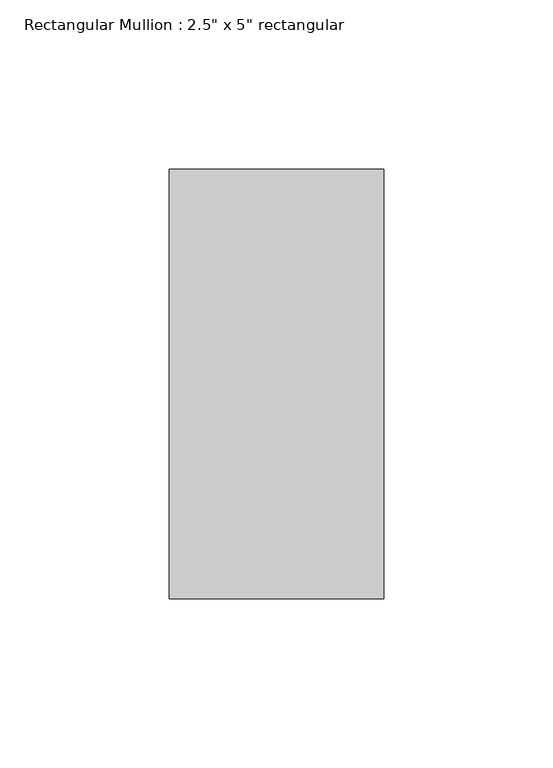
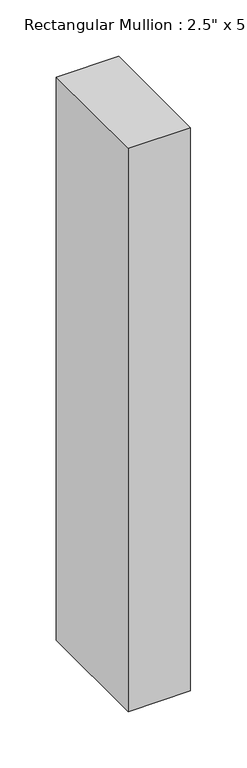
"""IFC4 building model written with IfcOpenShell, lengths in millimetres: member geometry."""

from ifc_helpers import new_model, si_unit, frame, origin, place, context, project, spatial, polyline, outline, extrude, source, transform, mapped, element, save


def member_cffb459a(model_context):
    return source(origin(), model_context, "Body", "SweptSolid", [
        extrude(outline(polyline([(31.75, 63.5), (31.75, -63.5), (-31.75, -63.5), (-31.75, 63.5), (31.75, 63.5)])), frame((0.0, 0.0, -609.1997047), z_axis=(0.0, 0.0, 1.0), x_axis=(1.0, 0.0, 0.0)), (0.0, 0.0, 1.0), 609.1997047),
    ])


if __name__ == "__main__":
    model = new_model("IFC4")
    model_context = context("Model", 3, world=origin())
    ifc_project = project(units=[si_unit("LENGTHUNIT", "METRE", prefix="MILLI")], contexts=[model_context])
    site = spatial("IfcSite", under=ifc_project)
    building = spatial("IfcBuilding", under=site)
    placement = place(None, origin())
    member_shape = member_cffb459a(model_context)
    element("IfcMember", 1, ObjectType="Rectangular Mullion : 2.5\" x 5\" rectangular", at=placement, inside=building, context=model_context, shape_type="MappedRepresentation", body=[
        mapped(member_shape, transform((0.0, 0.0, 0.0), x_axis=(1.0, 0.0, 0.0), y_axis=(0.0, 1.0, 0.0), z_axis=(0.0, 0.0, 1.0))),
    ])
    save(model, "model.ifc")

# Revit data of these elements
# Type "Rectangular Mullion : 2.5\" x 5\" rectangular"
#   built-in parameter 1007304 = 0.416667 (stored number, unit not read)
#   built-in parameter 1007301 = 0.104167 (stored number, unit not read)
#   built-in parameter 1007300 = 0.104167 (stored number, unit not read)
# Element 1 (IfcMember, "Rectangular Mullion : 2.5\" x 5\" rectangular")
#   Materials on its faces: "Aluminum"
# Materials
#   "Aluminum": class "Metal", colour RGB 247 247 247, transparency 0, Description = "Aluminum 6061", Cost = 0
